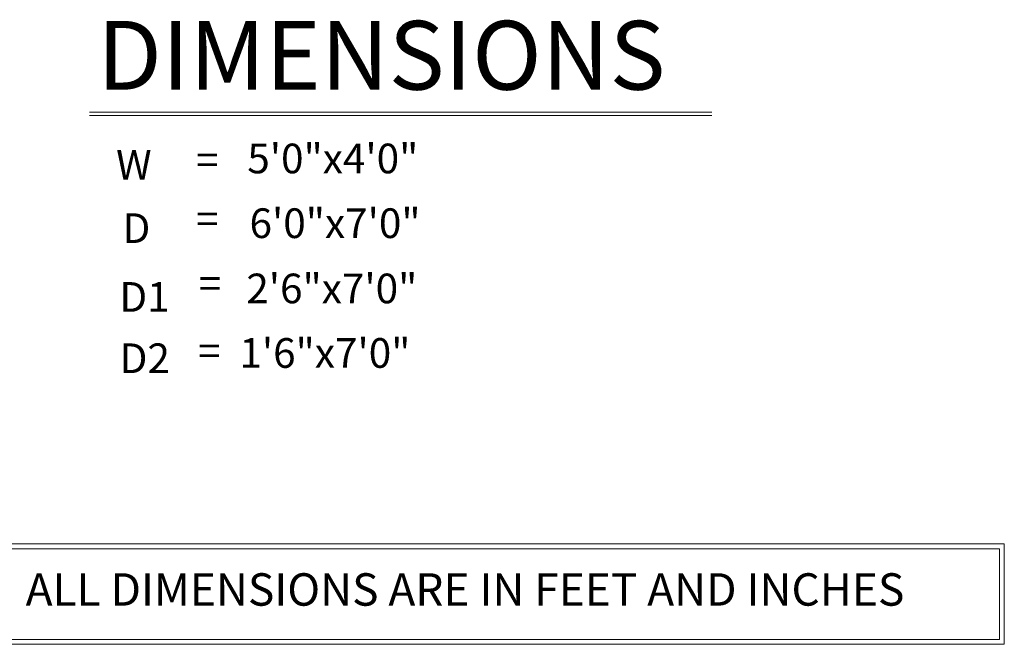
# Model space of a CAD drawing. Units: inches. Extents: x 1953 to 3378, y 1378 to 2530.
# Tile 5 of 5: x 2782 to 3378, y 1627 to 2006. Entities that reach past the tile are written whole.
import ezdxf

# ---------------------------------------------------------------- set-up
doc = ezdxf.new("R2010")
doc.units = ezdxf.units.IN
doc.layers.add('A-ANNO-SCHD', color=7, linetype='Continuous', lineweight=18)
doc.layers.add('A-ANNO-TEXT', color=7, linetype='Continuous', lineweight=18)
doc.styles.get("Standard").update_dxf_attribs({"font": 'arial.ttf'})

msp = doc.modelspace()

# ---------------------------------------------------------------- linework, layer by layer
at = {"layer": 'A-ANNO-SCHD'}
for p, q in [((2823.9, 1949.93), (3201.12, 1949.93)), ((2823.9, 1947.93), (3201.12, 1947.93))]:
    msp.add_line(p, q, dxfattribs=at)
at = {"layer": 'A-ANNO-TEXT'}
for points in [[(2766.11, 1688.1), (3378.35, 1688.1), (3378.35, 1627.13), (2766.11, 1627.13)], [(2769.11, 1685.1), (3375.35, 1685.1), (3375.35, 1630.13), (2769.11, 1630.13)]]:
    msp.add_lwpolyline(points, close=True, dxfattribs=at)

# ---------------------------------------------------------------- texts
at = {"layer": 'A-ANNO-SCHD'}
for s, height, p in [('DIMENSIONS', 41.692, (2828.55, 1963.52)), ('5\'0"x4\'0"', 18, (2919.48, 1912.78)), ('W', 18, (2839.93, 1908.96)), ('=', 18, (2888.37, 1911.86)), ('6\'0"x7\'0"', 18, (2920.83, 1873.53)), ('D', 18, (2843.82, 1870.51)), ('=', 18, (2888.37, 1876.14)), ('2\'6"x7\'0"', 18, (2918.87, 1833.95)), ('D1', 18, (2841.92, 1828.81)), ('=', 18, (2890.09, 1836.97)), ('D2', 18, (2842.05, 1791.62)), ('=', 18, (2889.66, 1796.08)), ('1\'6"x7\'0"', 18, (2914.67, 1794.82))]:
    msp.add_text(s, height=height, dxfattribs=at).set_placement(p)
at = {"layer": 'A-ANNO-TEXT'}
msp.add_text('ALL DIMENSIONS ARE IN FEET AND INCHES', height=19.6626, dxfattribs=at).set_placement((2785.13, 1650.56))

doc.saveas('drawing.dxf')
